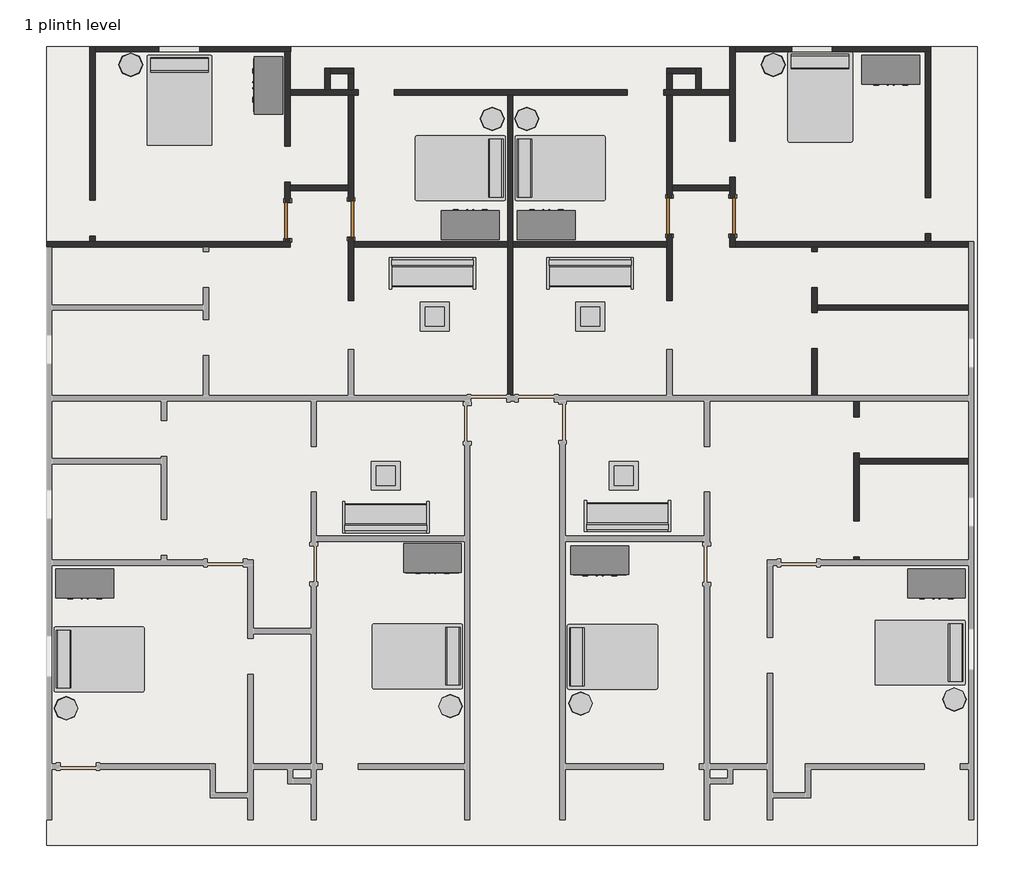
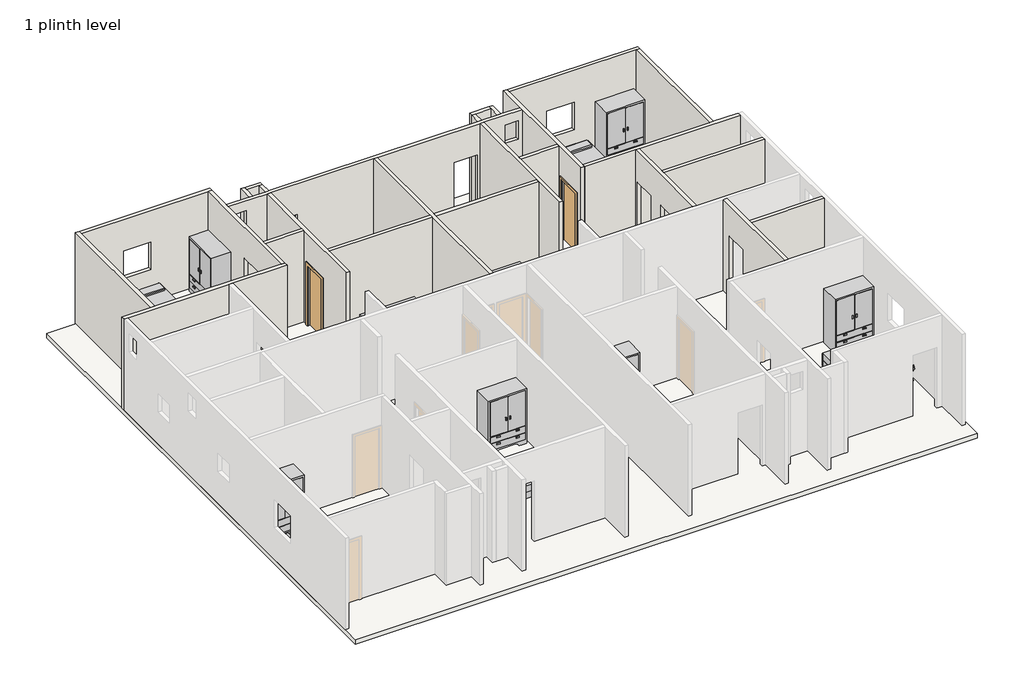
# One storey, part 2 of 2: 32 furniture elements, 26 walls, 4 doors, 1 slab.
"""IFC4 building model written with IfcOpenShell, lengths in millimetres."""

from ifc_helpers import new_model, si_unit, frame, origin, place, context, project, spatial, polyline, outline, extrude, faceted_brep, transform, mapped, element, save
from components import door_f2b275c1, door_d8f5dbb5, furniture_52ef1662, furniture_57f9710a, furniture_d3665cec, furniture_9d41381f, furniture_82e269c4

model = new_model("IFC4")

# Units and contexts
model_context = context("Model", 3, world=origin())
ifc_project = project(units=[si_unit("LENGTHUNIT", "METRE", prefix="MILLI")], contexts=[model_context])

# Site, building, storey
site = spatial("IfcSite", under=ifc_project)
building = spatial("IfcBuilding", under=site)
storey = spatial("IfcBuildingStorey", under=building, Name="1 plinth level", Elevation=457.2)

# Doors
placement = place(None, origin())
door_shape = door_f2b275c1(model_context)
element("IfcDoor", 1, ObjectType="Single-Flush : 30\" x 80\"", at=placement, inside=storey, context=model_context, shape_type="MappedRepresentation", body=[
    mapped(door_shape, transform((-9758.6269874, 1511.4935601, 457.2), x_axis=(0.0, -1.0, 0.0), y_axis=(1.0, 0.0, 0.0), z_axis=(0.0, 0.0, 1.0))),
])
element("IfcDoor", 2, ObjectType="Single-Flush : 30\" x 80\"", at=placement, inside=storey, context=model_context, shape_type="MappedRepresentation", body=[
    mapped(door_shape, transform((-1689.6343188, 1600.3935601, 457.2), x_axis=(0.0, -1.0, 0.0), y_axis=(1.0, 0.0, 0.0), z_axis=(0.0, 0.0, 1.0))),
])
door_2_shape = door_d8f5dbb5(model_context)
element("IfcDoor", 3, ObjectType="Single-Flush : 30\" x 80\"", at=placement, inside=storey, context=model_context, shape_type="MappedRepresentation", body=[
    mapped(door_2_shape, transform((-8420.6343188, 1536.8935601, 457.2), x_axis=(0.0, -1.0, 0.0), y_axis=(1.0, 0.0, 0.0), z_axis=(0.0, 0.0, 1.0))),
])
element("IfcDoor", 4, ObjectType="Single-Flush : 30\" x 80\"", at=placement, inside=storey, context=model_context, shape_type="MappedRepresentation", body=[
    mapped(door_2_shape, transform((-356.1343188, 1600.3935601, 457.2), x_axis=(0.0, -1.0, 0.0), y_axis=(1.0, 0.0, 0.0), z_axis=(0.0, 0.0, 1.0))),
])

# Furniture
furniture_shape = furniture_52ef1662(model_context)
element("IfcFurniture", 5, ObjectType="Bed-Standard : Double 54\" x 75\"", at=placement, inside=storey, context=model_context, shape_type="MappedRepresentation", body=[
    mapped(furniture_shape, transform((-12316.115512, 4097.0886421, 457.2), x_axis=(1.0, 0.0, 0.0), y_axis=(0.0, 1.0, 0.0), z_axis=(0.0, 0.0, 1.0))),
])
element("IfcFurniture", 6, ObjectType="Bed-Standard : Double 54\" x 75\"", at=placement, inside=storey, context=model_context, shape_type="MappedRepresentation", body=[
    mapped(furniture_shape, transform((-6063.6392368, 2886.3142767, 457.2), x_axis=(0.0, -1.0, 0.0), y_axis=(1.0, 0.0, 0.0), z_axis=(0.0, 0.0, 1.0))),
])
element("IfcFurniture", 7, ObjectType="Bed-Standard : Double 54\" x 75\"", at=placement, inside=storey, context=model_context, shape_type="MappedRepresentation", body=[
    mapped(furniture_shape, transform((-4046.6294008, 2343.3372275, 457.2), x_axis=(0.0, 1.0, 0.0), y_axis=(-1.0, 0.0, 0.0), z_axis=(0.0, 0.0, 1.0))),
])
element("IfcFurniture", 8, ObjectType="Bed-Standard : Double 54\" x 75\"", at=placement, inside=storey, context=model_context, shape_type="MappedRepresentation", body=[
    mapped(furniture_shape, transform((1220.2271566, 4166.9386421, 457.2), x_axis=(1.0, 0.0, 0.0), y_axis=(0.0, 1.0, 0.0), z_axis=(0.0, 0.0, 1.0))),
])
element("IfcFurniture", 9, ObjectType="Bed-Standard : Double 54\" x 75\"", at=placement, inside=storey, context=model_context, shape_type="MappedRepresentation", body=[
    mapped(furniture_shape, transform((-13787.5294008, -8037.3449645, 457.2), x_axis=(0.0, 1.0, 0.0), y_axis=(-1.0, 0.0, 0.0), z_axis=(0.0, 0.0, 1.0))),
])
element("IfcFurniture", 10, ObjectType="Bed-Standard : Double 54\" x 75\"", at=placement, inside=storey, context=model_context, shape_type="MappedRepresentation", body=[
    mapped(furniture_shape, transform((-6972.9182387, -7430.8679153, 457.2), x_axis=(0.0, -1.0, 0.0), y_axis=(1.0, 0.0, 0.0), z_axis=(0.0, 0.0, 1.0))),
])
element("IfcFurniture", 11, ObjectType="Bed-Standard : Double 54\" x 75\"", at=placement, inside=storey, context=model_context, shape_type="MappedRepresentation", body=[
    mapped(furniture_shape, transform((-2941.8986045, -7986.5449645, 457.2), x_axis=(0.0, 1.0, 0.0), y_axis=(-1.0, 0.0, 0.0), z_axis=(0.0, 0.0, 1.0))),
])
element("IfcFurniture", 12, ObjectType="Bed-Standard : Double 54\" x 75\"", at=placement, inside=storey, context=model_context, shape_type="MappedRepresentation", body=[
    mapped(furniture_shape, transform((3651.8607632, -7354.6679153, 457.2), x_axis=(0.0, -1.0, 0.0), y_axis=(1.0, 0.0, 0.0), z_axis=(0.0, 0.0, 1.0))),
])
furniture_2_shape = furniture_57f9710a(model_context)
element("IfcFurniture", 13, ObjectType="Sofa : 72\"", at=placement, inside=storey, context=model_context, shape_type="MappedRepresentation", body=[
    mapped(furniture_2_shape, transform((-6771.3838124, 247.7394618, 457.2), x_axis=(1.0, 0.0, 0.0), y_axis=(0.0, 1.0, 0.0), z_axis=(0.0, 0.0, 1.0))),
])
element("IfcFurniture", 14, ObjectType="Sofa : 72\"", at=placement, inside=storey, context=model_context, shape_type="MappedRepresentation", body=[
    mapped(furniture_2_shape, transform((-3436.4048106, 247.7394618, 457.2), x_axis=(1.0, 0.0, 0.0), y_axis=(0.0, 1.0, 0.0), z_axis=(0.0, 0.0, 1.0))),
])
element("IfcFurniture", 15, ObjectType="Sofa : 72\"", at=placement, inside=storey, context=model_context, shape_type="MappedRepresentation", body=[
    mapped(furniture_2_shape, transform((-7613.663827, -4616.1523415, 457.2), x_axis=(-1.0, 0.0, 0.0), y_axis=(0.0, -1.0, 0.0), z_axis=(0.0, 0.0, 1.0))),
])
element("IfcFurniture", 16, ObjectType="Sofa : 72\"", at=placement, inside=storey, context=model_context, shape_type="MappedRepresentation", body=[
    mapped(furniture_2_shape, transform((-2508.4330307, -4590.7523415, 457.2), x_axis=(-1.0, 0.0, 0.0), y_axis=(0.0, -1.0, 0.0), z_axis=(0.0, 0.0, 1.0))),
])
furniture_3_shape = furniture_d3665cec(model_context)
element("IfcFurniture", 17, ObjectType="Table-Coffee : 24\" x 24\" x 24\"", at=placement, inside=storey, context=model_context, shape_type="MappedRepresentation", body=[
    mapped(furniture_3_shape, transform((-6668.4790873, -615.7175177, 457.2), x_axis=(1.0, 0.0, 0.0), y_axis=(0.0, 1.0, 0.0), z_axis=(0.0, 0.0, 1.0))),
])
element("IfcFurniture", 18, ObjectType="Table-Coffee : 24\" x 24\" x 24\"", at=placement, inside=storey, context=model_context, shape_type="MappedRepresentation", body=[
    mapped(furniture_3_shape, transform((-3384.3000855, -615.7175177, 457.2), x_axis=(1.0, 0.0, 0.0), y_axis=(0.0, 1.0, 0.0), z_axis=(0.0, 0.0, 1.0))),
])
element("IfcFurniture", 19, ObjectType="Table-Coffee : 24\" x 24\" x 24\"", at=placement, inside=storey, context=model_context, shape_type="MappedRepresentation", body=[
    mapped(furniture_3_shape, transform((-7702.3000855, -3981.2175177, 457.2), x_axis=(1.0, 0.0, 0.0), y_axis=(0.0, 1.0, 0.0), z_axis=(0.0, 0.0, 1.0))),
])
element("IfcFurniture", 20, ObjectType="Table-Coffee : 24\" x 24\" x 24\"", at=placement, inside=storey, context=model_context, shape_type="MappedRepresentation", body=[
    mapped(furniture_3_shape, transform((-2673.1000855, -3981.2175177, 457.2), x_axis=(1.0, 0.0, 0.0), y_axis=(0.0, 1.0, 0.0), z_axis=(0.0, 0.0, 1.0))),
])
furniture_4_shape = furniture_9d41381f(model_context)
element("IfcFurniture", 21, ObjectType="Table-Trio End : 20\" Diameter", at=placement, inside=storey, context=model_context, shape_type="MappedRepresentation", body=[
    mapped(furniture_4_shape, transform((-13075.1843188, 4800.7935601, 457.2), x_axis=(1.0, 0.0, 0.0), y_axis=(0.0, 1.0, 0.0), z_axis=(0.0, 0.0, 1.0))),
])
element("IfcFurniture", 22, ObjectType="Table-Trio End : 20\" Diameter", at=placement, inside=storey, context=model_context, shape_type="MappedRepresentation", body=[
    mapped(furniture_4_shape, transform((-5436.1343188, 3657.7935601, 457.2), x_axis=(1.0, 0.0, 0.0), y_axis=(0.0, 1.0, 0.0), z_axis=(0.0, 0.0, 1.0))),
])
element("IfcFurniture", 23, ObjectType="Table-Trio End : 20\" Diameter", at=placement, inside=storey, context=model_context, shape_type="MappedRepresentation", body=[
    mapped(furniture_4_shape, transform((-4706.6059618, 3657.7935601, 457.2), x_axis=(1.0, 0.0, 0.0), y_axis=(0.0, 1.0, 0.0), z_axis=(0.0, 0.0, 1.0))),
])
element("IfcFurniture", 24, ObjectType="Table-Trio End : 20\" Diameter", at=placement, inside=storey, context=model_context, shape_type="MappedRepresentation", body=[
    mapped(furniture_4_shape, transform((501.1156812, 4800.7935601, 457.2), x_axis=(1.0, 0.0, 0.0), y_axis=(0.0, 1.0, 0.0), z_axis=(0.0, 0.0, 1.0))),
])
element("IfcFurniture", 25, ObjectType="Table-Trio End : 20\" Diameter", at=placement, inside=storey, context=model_context, shape_type="MappedRepresentation", body=[
    mapped(furniture_4_shape, transform((4330.1656812, -8616.7564399, 457.2), x_axis=(1.0, 0.0, 0.0), y_axis=(0.0, 1.0, 0.0), z_axis=(0.0, 0.0, 1.0))),
])
element("IfcFurniture", 26, ObjectType="Table-Trio End : 20\" Diameter", at=placement, inside=storey, context=model_context, shape_type="MappedRepresentation", body=[
    mapped(furniture_4_shape, transform((-3569.2343188, -8702.0106007, 457.2), x_axis=(1.0, 0.0, 0.0), y_axis=(0.0, 1.0, 0.0), z_axis=(0.0, 0.0, 1.0))),
])
element("IfcFurniture", 27, ObjectType="Table-Trio End : 20\" Diameter", at=placement, inside=storey, context=model_context, shape_type="MappedRepresentation", body=[
    mapped(furniture_4_shape, transform((-6320.0133206, -8756.4564399, 457.2), x_axis=(1.0, 0.0, 0.0), y_axis=(0.0, 1.0, 0.0), z_axis=(0.0, 0.0, 1.0))),
])
element("IfcFurniture", 28, ObjectType="Table-Trio End : 20\" Diameter", at=placement, inside=storey, context=model_context, shape_type="MappedRepresentation", body=[
    mapped(furniture_4_shape, transform((-14440.4343188, -8800.9064399, 457.2), x_axis=(1.0, 0.0, 0.0), y_axis=(0.0, 1.0, 0.0), z_axis=(0.0, 0.0, 1.0))),
])
furniture_5_shape = furniture_82e269c4(model_context)
element("IfcFurniture", 29, ObjectType="Wardrobe : 48\" x 72\" x 24\"", at=placement, inside=storey, context=model_context, shape_type="MappedRepresentation", body=[
    mapped(furniture_5_shape, transform((-9581.2881778, 4098.2324922, 457.2), x_axis=(0.0, -1.0, 0.0), y_axis=(1.0, 0.0, 0.0), z_axis=(0.0, 0.0, 1.0))),
])
element("IfcFurniture", 30, ObjectType="Wardrobe : 48\" x 72\" x 24\"", at=placement, inside=storey, context=model_context, shape_type="MappedRepresentation", body=[
    mapped(furniture_5_shape, transform((-6168.8775786, 826.1547505, 457.2), x_axis=(-1.0, 0.0, 0.0), y_axis=(0.0, -1.0, 0.0), z_axis=(0.0, 0.0, 1.0))),
])
element("IfcFurniture", 31, ObjectType="Wardrobe : 48\" x 72\" x 24\"", at=placement, inside=storey, context=model_context, shape_type="MappedRepresentation", body=[
    mapped(furniture_5_shape, transform((-4562.3275786, 826.1547505, 457.2), x_axis=(-1.0, 0.0, 0.0), y_axis=(0.0, -1.0, 0.0), z_axis=(0.0, 0.0, 1.0))),
])
element("IfcFurniture", 32, ObjectType="Wardrobe : 48\" x 72\" x 24\"", at=placement, inside=storey, context=model_context, shape_type="MappedRepresentation", body=[
    mapped(furniture_5_shape, transform((3253.158941, 5282.9323697, 457.2), x_axis=(1.0, 0.0, 0.0), y_axis=(0.0, 1.0, 0.0), z_axis=(0.0, 0.0, 1.0))),
])
element("IfcFurniture", 33, ObjectType="Wardrobe : 48\" x 72\" x 24\"", at=placement, inside=storey, context=model_context, shape_type="MappedRepresentation", body=[
    mapped(furniture_5_shape, transform((4218.358941, -5575.5676303, 457.2), x_axis=(1.0, 0.0, 0.0), y_axis=(0.0, 1.0, 0.0), z_axis=(0.0, 0.0, 1.0))),
])
element("IfcFurniture", 34, ObjectType="Wardrobe : 48\" x 72\" x 24\"", at=placement, inside=storey, context=model_context, shape_type="MappedRepresentation", body=[
    mapped(furniture_5_shape, transform((-2893.641059, -5086.6176303, 457.2), x_axis=(1.0, 0.0, 0.0), y_axis=(0.0, 1.0, 0.0), z_axis=(0.0, 0.0, 1.0))),
])
element("IfcFurniture", 35, ObjectType="Wardrobe : 48\" x 72\" x 24\"", at=placement, inside=storey, context=model_context, shape_type="MappedRepresentation", body=[
    mapped(furniture_5_shape, transform((-6431.8200608, -5042.1676303, 457.2), x_axis=(1.0, 0.0, 0.0), y_axis=(0.0, 1.0, 0.0), z_axis=(0.0, 0.0, 1.0))),
])
element("IfcFurniture", 36, ObjectType="Wardrobe : 48\" x 72\" x 24\"", at=placement, inside=storey, context=model_context, shape_type="MappedRepresentation", body=[
    mapped(furniture_5_shape, transform((-13777.541059, -5575.5676303, 457.2), x_axis=(1.0, 0.0, 0.0), y_axis=(0.0, 1.0, 0.0), z_axis=(0.0, 0.0, 1.0))),
])

# Slab
element("IfcSlab", 37, ObjectType="6\"", at=placement, inside=storey, context=model_context, shape_type="SweptSolid", body=[
    extrude(outline(polyline([(-14853.1843188, -11697.2008638), (-14853.1843188, 5188.1435601), (4816.0294854, 5188.1435601), (4816.0294854, -11697.2008638), (-14853.1843188, -11697.2008638)])), frame((0.0, 0.0, 304.8), z_axis=(0.0, 0.0, 1.0), x_axis=(1.0, 0.0, 0.0)), (0.0, 0.0, 1.0), 152.4),
])

# Walls
element("IfcWall", 38, ObjectType="wall-4.5\"", at=placement, inside=storey, context=model_context, shape_type="Brep", body=[
    faceted_brep([(-13824.4843188, 5073.8435601, 457.2), (-9815.7769874, 5073.8435601, 457.2), (-9701.4769874, 5073.8435601, 457.2), (-9696.9843188, 5073.8435601, 457.2), (-9696.9843188, 5073.8435601, 3505.2), (-9701.4769874, 5073.8435601, 3505.2), (-9815.7769874, 5073.8435601, 3505.2), (-13824.4843188, 5073.8435601, 3505.2), (-11621.0343188, 5073.8435601, 2438.4), (-11621.0343188, 5073.8435601, 1524.0), (-12484.6343188, 5073.8435601, 1524.0), (-12484.6343188, 5073.8435601, 2438.4), (-13824.4843188, 5188.1435601, 457.2), (-13824.4843188, 5188.1435601, 3505.2), (-9696.9843188, 5188.1435601, 3505.2), (-9696.9843188, 5188.1435601, 457.2), (-11621.0343188, 5188.1435601, 2438.4), (-12484.6343188, 5188.1435601, 2438.4), (-12484.6343188, 5188.1435601, 1524.0), (-11621.0343188, 5188.1435601, 1524.0)], [[[0, 1, 2, 3, 4, 5, 6, 7], [8, 9, 10, 11]], [[12, 13, 14, 15], [16, 17, 18, 19]], [[3, 2, 1, 0, 12, 15]], [[4, 3, 15, 14]], [[7, 6, 5, 4, 14, 13]], [[0, 7, 13, 12]], [[9, 8, 16, 19]], [[10, 9, 19, 18]], [[11, 10, 18, 17]], [[8, 11, 17, 16]]]),
])
element("IfcWall", 39, ObjectType="wall-4.5\"", at=placement, inside=storey, context=model_context, shape_type="Brep", body=[
    faceted_brep([(-9815.7769874, 2324.2935601, 2489.2), (-9815.7769874, 2324.2935601, 457.2), (-9815.7769874, 1892.4935601, 457.2), (-9815.7769874, 1892.4935601, 2489.2), (-9815.7769874, 1130.4935601, 2489.2), (-9815.7769874, 1130.4935601, 457.2), (-9815.7769874, 1060.6435601, 457.2), (-9815.7769874, 1060.6435601, 3505.2), (-9815.7769874, 5073.8435601, 3505.2), (-9815.7769874, 5073.8435601, 457.2), (-9815.7769874, 3086.2935601, 457.2), (-9815.7769874, 3086.2935601, 2489.2), (-9701.4769874, 1892.4935601, 457.2), (-9701.4769874, 2140.1435601, 457.2), (-9701.4769874, 2254.4435601, 457.2), (-9701.4769874, 2324.2935601, 457.2), (-9701.4769874, 2324.2935601, 2489.2), (-9701.4769874, 3086.2935601, 2489.2), (-9701.4769874, 3086.2935601, 457.2), (-9701.4769874, 4159.4435601, 457.2), (-9701.4769874, 4273.7435601, 457.2), (-9701.4769874, 5073.8435601, 457.2), (-9701.4769874, 5073.8435601, 3505.2), (-9701.4769874, 4273.7435601, 3505.2), (-9701.4769874, 4159.4435601, 3505.2), (-9701.4769874, 2254.4435601, 3505.2), (-9701.4769874, 2140.1435601, 3505.2), (-9701.4769874, 1060.6435601, 3505.2), (-9701.4769874, 1060.6435601, 457.2), (-9701.4769874, 1130.4935601, 457.2), (-9701.4769874, 1130.4935601, 2489.2), (-9701.4769874, 1892.4935601, 2489.2)], [[[0, 1, 2, 3, 4, 5, 6, 7, 8, 9, 10, 11]], [[12, 13, 14, 15, 16, 17, 18, 19, 20, 21, 22, 23, 24, 25, 26, 27, 28, 29, 30, 31]], [[28, 6, 5, 29]], [[10, 9, 21, 20, 19, 18]], [[2, 1, 15, 14, 13, 12]], [[8, 7, 27, 26, 25, 24, 23, 22]], [[7, 6, 28, 27]], [[9, 8, 22, 21]], [[4, 30, 29, 5]], [[30, 4, 3, 31]], [[31, 3, 2, 12]], [[16, 15, 1, 0]], [[17, 16, 0, 11]], [[18, 17, 11, 10]]]),
])
element("IfcWall", 40, ObjectType="wall-4.5\"", at=placement, inside=storey, context=model_context, shape_type="Brep", body=[
    faceted_brep([(-9701.4769874, 1060.6435601, 457.2), (-9815.7769874, 1060.6435601, 457.2), (-13824.4843188, 1060.6435601, 457.2), (-13938.7843188, 1060.6435601, 457.2), (-14853.1843188, 1060.6435601, 457.2), (-14853.1843188, 1060.6435601, 3505.2), (-13938.7843188, 1060.6435601, 3505.2), (-13824.4843188, 1060.6435601, 3505.2), (-9815.7769874, 1060.6435601, 3505.2), (-9701.4769874, 1060.6435601, 3505.2), (-9701.4769874, 946.3435601, 457.2), (-9701.4769874, 946.3435601, 3505.2), (-11424.1843188, 946.3435601, 3505.2), (-11538.4843188, 946.3435601, 3505.2), (-14738.8843188, 946.3435601, 3505.2), (-14853.1843188, 946.3435601, 3505.2), (-14853.1843188, 946.3435601, 457.2), (-14738.8843188, 946.3435601, 457.2), (-11538.4843188, 946.3435601, 457.2), (-11424.1843188, 946.3435601, 457.2)], [[[0, 1, 2, 3, 4, 5, 6, 7, 8, 9]], [[10, 11, 12, 13, 14, 15, 16, 17, 18, 19]], [[4, 3, 2, 1, 0, 10, 19, 18, 17, 16]], [[9, 8, 7, 6, 5, 15, 14, 13, 12, 11]], [[0, 9, 11, 10]], [[5, 4, 16, 15]]]),
])
element("IfcWall", 41, ObjectType="wall-4.5\"", at=placement, inside=storey, context=model_context, shape_type="Brep", body=[
    faceted_brep([(-13938.7843188, 1181.2935601, 2489.2), (-13938.7843188, 1181.2935601, 457.2), (-13938.7843188, 1060.6435601, 457.2), (-13938.7843188, 1060.6435601, 3505.2), (-13938.7843188, 5188.1435601, 3505.2), (-13938.7843188, 5188.1435601, 457.2), (-13938.7843188, 1943.2935601, 457.2), (-13938.7843188, 1943.2935601, 2489.2), (-13824.4843188, 1060.6435601, 457.2), (-13824.4843188, 1181.2935601, 457.2), (-13824.4843188, 1181.2935601, 2489.2), (-13824.4843188, 1943.2935601, 2489.2), (-13824.4843188, 1943.2935601, 457.2), (-13824.4843188, 5073.8435601, 457.2), (-13824.4843188, 5188.1435601, 457.2), (-13824.4843188, 5188.1435601, 3505.2), (-13824.4843188, 5073.8435601, 3505.2), (-13824.4843188, 1060.6435601, 3505.2)], [[[0, 1, 2, 3, 4, 5, 6, 7]], [[8, 9, 10, 11, 12, 13, 14, 15, 16, 17]], [[6, 5, 14, 13, 12]], [[2, 1, 9, 8]], [[4, 3, 17, 16, 15]], [[3, 2, 8, 17]], [[5, 4, 15, 14]], [[10, 9, 1, 0]], [[11, 10, 0, 7]], [[12, 11, 7, 6]]]),
])
element("IfcWall", 42, ObjectType="wall-4.5\"", at=placement, inside=storey, context=model_context, shape_type="Brep", body=[
    faceted_brep([(-9701.4769874, 4159.4435601, 457.2), (-8477.7843188, 4159.4435601, 457.2), (-8363.4843188, 4159.4435601, 457.2), (-8266.3769874, 4159.4435601, 457.2), (-8266.3769874, 4159.4435601, 2489.2), (-7504.3769874, 4159.4435601, 2489.2), (-7504.3769874, 4159.4435601, 457.2), (-5112.2843188, 4159.4435601, 457.2), (-4997.9843188, 4159.4435601, 457.2), (-2578.6343188, 4159.4435601, 457.2), (-2578.6343188, 4159.4435601, 2489.2), (-1816.6343188, 4159.4435601, 2489.2), (-1816.6343188, 4159.4435601, 457.2), (-1746.7843188, 4159.4435601, 457.2), (-1632.4843188, 4159.4435601, 457.2), (-414.0059618, 4159.4435601, 457.2), (-414.0059618, 4159.4435601, 3505.2), (-1632.4843188, 4159.4435601, 3505.2), (-1746.7843188, 4159.4435601, 3505.2), (-4997.9843188, 4159.4435601, 3505.2), (-5112.2843188, 4159.4435601, 3505.2), (-8363.4843188, 4159.4435601, 3505.2), (-8477.7843188, 4159.4435601, 3505.2), (-9701.4769874, 4159.4435601, 3505.2), (-9134.0806531, 4159.4435601, 3175.0), (-9134.0806531, 4159.4435601, 2565.4), (-9540.4806531, 4159.4435601, 2565.4), (-9540.4806531, 4159.4435601, 3175.0), (-543.8201403, 4159.4435601, 3175.0), (-543.8201403, 4159.4435601, 2565.4), (-950.2201403, 4159.4435601, 2565.4), (-950.2201403, 4159.4435601, 3175.0), (-8266.3769874, 4273.7435601, 2489.2), (-8266.3769874, 4273.7435601, 457.2), (-8361.6269874, 4273.7435601, 457.2), (-8475.9269874, 4273.7435601, 457.2), (-8858.7843188, 4273.7435601, 457.2), (-8973.0843188, 4273.7435601, 457.2), (-9701.4769874, 4273.7435601, 457.2), (-9701.4769874, 4273.7435601, 3505.2), (-8973.0843188, 4273.7435601, 3505.2), (-8858.7843188, 4273.7435601, 3505.2), (-8475.9269874, 4273.7435601, 3505.2), (-8361.6269874, 4273.7435601, 3505.2), (-1746.7843188, 4273.7435601, 3505.2), (-1632.4843188, 4273.7435601, 3505.2), (-1137.1843188, 4273.7435601, 3505.2), (-1022.8843188, 4273.7435601, 3505.2), (-414.0059618, 4273.7435601, 3505.2), (-414.0059618, 4273.7435601, 457.2), (-1022.8843188, 4273.7435601, 457.2), (-1137.1843188, 4273.7435601, 457.2), (-1632.4843188, 4273.7435601, 457.2), (-1746.7843188, 4273.7435601, 457.2), (-1816.6343188, 4273.7435601, 457.2), (-1816.6343188, 4273.7435601, 2489.2), (-2578.6343188, 4273.7435601, 2489.2), (-2578.6343188, 4273.7435601, 457.2), (-7504.3769874, 4273.7435601, 457.2), (-7504.3769874, 4273.7435601, 2489.2), (-9134.0806531, 4273.7435601, 3175.0), (-9540.4806531, 4273.7435601, 3175.0), (-9540.4806531, 4273.7435601, 2565.4), (-9134.0806531, 4273.7435601, 2565.4), (-543.8201403, 4273.7435601, 3175.0), (-950.2201403, 4273.7435601, 3175.0), (-950.2201403, 4273.7435601, 2565.4), (-543.8201403, 4273.7435601, 2565.4)], [[[0, 1, 2, 3, 4, 5, 6, 7, 8, 9, 10, 11, 12, 13, 14, 15, 16, 17, 18, 19, 20, 21, 22, 23], [24, 25, 26, 27], [28, 29, 30, 31]], [[32, 33, 34, 35, 36, 37, 38, 39, 40, 41, 42, 43, 44, 45, 46, 47, 48, 49, 50, 51, 52, 53, 54, 55, 56, 57, 58, 59], [60, 61, 62, 63], [64, 65, 66, 67]], [[15, 14, 13, 12, 54, 53, 52, 51, 50, 49]], [[58, 57, 9, 8, 7, 6]], [[38, 37, 36, 35, 34, 33, 3, 2, 1, 0]], [[16, 15, 49, 48]], [[23, 22, 21, 20, 19, 18, 17, 16, 48, 47, 46, 45, 44, 43, 42, 41, 40, 39]], [[0, 23, 39, 38]], [[55, 54, 12, 11]], [[56, 55, 11, 10]], [[57, 56, 10, 9]], [[4, 3, 33, 32]], [[5, 4, 32, 59]], [[6, 5, 59, 58]], [[25, 24, 60, 63]], [[26, 25, 63, 62]], [[27, 26, 62, 61]], [[24, 27, 61, 60]], [[29, 28, 64, 67]], [[30, 29, 67, 66]], [[31, 30, 66, 65]], [[28, 31, 65, 64]]]),
])
element("IfcWall", 43, ObjectType="wall-4.5\"", at=placement, inside=storey, context=model_context, shape_type="Brep", body=[
    faceted_brep([(-8858.7843188, 4273.7435601, 457.2), (-8858.7843188, 4616.6435601, 457.2), (-8858.7843188, 4730.9435601, 457.2), (-8858.7843188, 4730.9435601, 3505.2), (-8858.7843188, 4616.6435601, 3505.2), (-8858.7843188, 4273.7435601, 3505.2), (-8973.0843188, 4273.7435601, 457.2), (-8973.0843188, 4273.7435601, 3505.2), (-8973.0843188, 4730.9435601, 3505.2), (-8973.0843188, 4730.9435601, 457.2)], [[[0, 1, 2, 3, 4, 5]], [[6, 7, 8, 9]], [[2, 1, 0, 6, 9]], [[5, 4, 3, 8, 7]], [[0, 5, 7, 6]], [[3, 2, 9, 8]]]),
])
element("IfcWall", 44, ObjectType="wall-4.5\"", at=placement, inside=storey, context=model_context, shape_type="SweptSolid", body=[
    extrude(outline(polyline([(-8361.6269874, 4616.6435601), (-8361.6269874, 4273.7435601), (-8475.9269874, 4273.7435601), (-8475.9269874, 4616.6435601), (-8361.6269874, 4616.6435601)])), frame((0.0, 0.0, 457.2), z_axis=(0.0, 0.0, 1.0), x_axis=(1.0, 0.0, 0.0)), (0.0, 0.0, 1.0), 3048.0),
])
element("IfcWall", 45, ObjectType="wall-4.5\"", at=placement, inside=storey, context=model_context, shape_type="Brep", body=[
    faceted_brep([(-8361.6269874, 4730.9435601, 457.2), (-8858.7843188, 4730.9435601, 457.2), (-8858.7843188, 4730.9435601, 3505.2), (-8361.6269874, 4730.9435601, 3505.2), (-8361.6269874, 4616.6435601, 457.2), (-8361.6269874, 4616.6435601, 3505.2), (-8475.9269874, 4616.6435601, 3505.2), (-8858.7843188, 4616.6435601, 3505.2), (-8858.7843188, 4616.6435601, 457.2), (-8475.9269874, 4616.6435601, 457.2)], [[[0, 1, 2, 3]], [[4, 5, 6, 7, 8, 9]], [[1, 0, 4, 9, 8]], [[3, 2, 7, 6, 5]], [[2, 1, 8, 7]], [[0, 3, 5, 4]]]),
])
element("IfcWall", 46, ObjectType="wall-4.5\"", at=placement, inside=storey, context=model_context, shape_type="Brep", body=[
    faceted_brep([(-8477.7843188, -179.1742479, 457.2), (-8477.7843188, -179.1742479, 3505.2), (-8477.7843188, 2140.1435601, 3505.2), (-8477.7843188, 2254.4435601, 3505.2), (-8477.7843188, 4159.4435601, 3505.2), (-8477.7843188, 4159.4435601, 457.2), (-8477.7843188, 2254.4435601, 457.2), (-8477.7843188, 2140.1435601, 457.2), (-8477.7843188, 1917.8935601, 457.2), (-8477.7843188, 1917.8935601, 2489.2), (-8477.7843188, 1155.8935601, 2489.2), (-8477.7843188, 1155.8935601, 457.2), (-8363.4843188, -179.1742479, 3505.2), (-8363.4843188, -179.1742479, 457.2), (-8363.4843188, 946.3435601, 457.2), (-8363.4843188, 1060.6435601, 457.2), (-8363.4843188, 1155.8935601, 457.2), (-8363.4843188, 1155.8935601, 2489.2), (-8363.4843188, 1917.8935601, 2489.2), (-8363.4843188, 1917.8935601, 457.2), (-8363.4843188, 4159.4435601, 457.2), (-8363.4843188, 4159.4435601, 3505.2), (-8363.4843188, 1060.6435601, 3505.2), (-8363.4843188, 946.3435601, 3505.2)], [[[0, 1, 2, 3, 4, 5, 6, 7, 8, 9, 10, 11]], [[12, 13, 14, 15, 16, 17, 18, 19, 20, 21, 22, 23]], [[13, 0, 11, 16, 15, 14]], [[5, 20, 19, 8, 7, 6]], [[1, 0, 13, 12]], [[4, 3, 2, 1, 12, 23, 22, 21]], [[5, 4, 21, 20]], [[10, 17, 16, 11]], [[17, 10, 9, 18]], [[18, 9, 8, 19]]]),
])
element("IfcWall", 47, ObjectType="wall-4.5\"", at=placement, inside=storey, context=model_context, shape_type="Brep", body=[
    faceted_brep([(-413.2843188, 5188.1435601, 457.2), (-413.2843188, 3187.8935601, 457.2), (-413.2843188, 3187.8935601, 2489.2), (-413.2843188, 2425.8935601, 2489.2), (-413.2843188, 2425.8935601, 457.2), (-413.2843188, 2254.4435601, 457.2), (-413.2843188, 2140.1435601, 457.2), (-413.2843188, 1981.3935601, 457.2), (-413.2843188, 1981.3935601, 2489.2), (-413.2843188, 1219.3935601, 2489.2), (-413.2843188, 1219.3935601, 457.2), (-413.2843188, 946.3435601, 457.2), (-413.2843188, 946.3435601, 3505.2), (-413.2843188, 2140.1435601, 3505.2), (-413.2843188, 2254.4435601, 3505.2), (-413.2843188, 5188.1435601, 3505.2), (-298.9843188, 3187.8935601, 2489.2), (-298.9843188, 3187.8935601, 457.2), (-298.9843188, 5073.8435601, 457.2), (-298.9843188, 5188.1435601, 457.2), (-298.9843188, 5188.1435601, 3505.2), (-298.9843188, 5073.8435601, 3505.2), (-298.9843188, 1060.6435601, 3505.2), (-298.9843188, 946.3435601, 3505.2), (-298.9843188, 946.3435601, 457.2), (-298.9843188, 1060.6435601, 457.2), (-298.9843188, 1219.3935601, 457.2), (-298.9843188, 1219.3935601, 2489.2), (-298.9843188, 1981.3935601, 2489.2), (-298.9843188, 1981.3935601, 457.2), (-298.9843188, 2425.8935601, 457.2), (-298.9843188, 2425.8935601, 2489.2)], [[[0, 1, 2, 3, 4, 5, 6, 7, 8, 9, 10, 11, 12, 13, 14, 15]], [[16, 17, 18, 19, 20, 21, 22, 23, 24, 25, 26, 27, 28, 29, 30, 31]], [[24, 11, 10, 26, 25]], [[30, 29, 7, 6, 5, 4]], [[19, 18, 17, 1, 0]], [[15, 14, 13, 12, 23, 22, 21, 20]], [[12, 11, 24, 23]], [[0, 15, 20, 19]], [[9, 27, 26, 10]], [[27, 9, 8, 28]], [[28, 8, 7, 29]], [[2, 1, 17, 16]], [[3, 2, 16, 31]], [[4, 3, 31, 30]]]),
])
element("IfcWall", 48, ObjectType="wall-4.5\"", at=placement, inside=storey, context=model_context, shape_type="Brep", body=[
    faceted_brep([(-298.9843188, 946.3435601, 457.2), (1313.9156812, 946.3435601, 457.2), (1428.2156812, 946.3435601, 457.2), (4628.6156812, 946.3435601, 457.2), (4628.6156812, 946.3435601, 3505.2), (1428.2156812, 946.3435601, 3505.2), (1313.9156812, 946.3435601, 3505.2), (-298.9843188, 946.3435601, 3505.2), (-298.9843188, 1060.6435601, 457.2), (-298.9843188, 1060.6435601, 3505.2), (3714.2156812, 1060.6435601, 3505.2), (3828.5156812, 1060.6435601, 3505.2), (4628.6156812, 1060.6435601, 3505.2), (4628.6156812, 1060.6435601, 457.2), (3828.5156812, 1060.6435601, 457.2), (3714.2156812, 1060.6435601, 457.2)], [[[0, 1, 2, 3, 4, 5, 6, 7]], [[8, 9, 10, 11, 12, 13, 14, 15]], [[3, 2, 1, 0, 8, 15, 14, 13]], [[7, 6, 5, 4, 12, 11, 10, 9]], [[0, 7, 9, 8]], [[4, 3, 13, 12]]]),
])
element("IfcWall", 49, ObjectType="wall-4.5\"", at=placement, inside=storey, context=model_context, shape_type="Brep", body=[
    faceted_brep([(-298.9843188, 5073.8435601, 457.2), (3714.2156812, 5073.8435601, 457.2), (3828.5156812, 5073.8435601, 457.2), (3828.5156812, 5073.8435601, 3505.2), (3714.2156812, 5073.8435601, 3505.2), (-298.9843188, 5073.8435601, 3505.2), (1752.0656812, 5073.8435601, 2438.4), (1752.0656812, 5073.8435601, 1524.0), (888.4656812, 5073.8435601, 1524.0), (888.4656812, 5073.8435601, 2438.4), (-298.9843188, 5188.1435601, 457.2), (-298.9843188, 5188.1435601, 3505.2), (3828.5156812, 5188.1435601, 3505.2), (3828.5156812, 5188.1435601, 457.2), (1752.0656812, 5188.1435601, 2438.4), (888.4656812, 5188.1435601, 2438.4), (888.4656812, 5188.1435601, 1524.0), (1752.0656812, 5188.1435601, 1524.0)], [[[0, 1, 2, 3, 4, 5], [6, 7, 8, 9]], [[10, 11, 12, 13], [14, 15, 16, 17]], [[2, 1, 0, 10, 13]], [[5, 4, 3, 12, 11]], [[0, 5, 11, 10]], [[3, 2, 13, 12]], [[7, 6, 14, 17]], [[8, 7, 17, 16]], [[9, 8, 16, 15]], [[6, 9, 15, 14]]]),
])
element("IfcWall", 50, ObjectType="wall-4.5\"", at=placement, inside=storey, context=model_context, shape_type="SweptSolid", body=[
    extrude(outline(polyline([(1232.0935601, 2489.2), (1232.0935601, 457.2), (1060.6435601, 457.2), (1060.6435601, 3505.2), (5073.8435601, 3505.2), (5073.8435601, 457.2), (1994.0935601, 457.2), (1994.0935601, 2489.2), (1232.0935601, 2489.2)])), frame((3714.2156812, 0.0, 0.0), z_axis=(1.0, 0.0, 0.0), x_axis=(0.0, 1.0, 0.0)), (0.0, 0.0, 1.0), 114.3),
])
element("IfcWall", 51, ObjectType="wall-4.5\"", at=placement, inside=storey, context=model_context, shape_type="SweptSolid", body=[
    extrude(outline(polyline([(-8477.7843188, 2140.1435601), (-9701.4769874, 2140.1435601), (-9701.4769874, 2254.4435601), (-8477.7843188, 2254.4435601), (-8477.7843188, 2140.1435601)])), frame((0.0, 0.0, 457.2), z_axis=(0.0, 0.0, 1.0), x_axis=(1.0, 0.0, 0.0)), (0.0, 0.0, 1.0), 3048.0),
])
element("IfcWall", 52, ObjectType="wall-4.5\"", at=placement, inside=storey, context=model_context, shape_type="SweptSolid", body=[
    extrude(outline(polyline([(-1632.4843188, 4616.6435601), (-1632.4843188, 4273.7435601), (-1746.7843188, 4273.7435601), (-1746.7843188, 4616.6435601), (-1632.4843188, 4616.6435601)])), frame((0.0, 0.0, 457.2), z_axis=(0.0, 0.0, 1.0), x_axis=(1.0, 0.0, 0.0)), (0.0, 0.0, 1.0), 3048.0),
])
element("IfcWall", 53, ObjectType="wall-4.5\"", at=placement, inside=storey, context=model_context, shape_type="Brep", body=[
    faceted_brep([(-1746.7843188, 4616.6435601, 457.2), (-1632.4843188, 4616.6435601, 457.2), (-1137.1843188, 4616.6435601, 457.2), (-1137.1843188, 4616.6435601, 3505.2), (-1632.4843188, 4616.6435601, 3505.2), (-1746.7843188, 4616.6435601, 3505.2), (-1746.7843188, 4730.9435601, 457.2), (-1746.7843188, 4730.9435601, 3505.2), (-1137.1843188, 4730.9435601, 3505.2), (-1137.1843188, 4730.9435601, 457.2)], [[[0, 1, 2, 3, 4, 5]], [[6, 7, 8, 9]], [[2, 1, 0, 6, 9]], [[5, 4, 3, 8, 7]], [[3, 2, 9, 8]], [[0, 5, 7, 6]]]),
])
element("IfcWall", 54, ObjectType="wall-4.5\"", at=placement, inside=storey, context=model_context, shape_type="Brep", body=[
    faceted_brep([(-1137.1843188, 4730.9435601, 457.2), (-1137.1843188, 4616.6435601, 457.2), (-1137.1843188, 4273.7435601, 457.2), (-1137.1843188, 4273.7435601, 3505.2), (-1137.1843188, 4616.6435601, 3505.2), (-1137.1843188, 4730.9435601, 3505.2), (-1022.8843188, 4730.9435601, 457.2), (-1022.8843188, 4730.9435601, 3505.2), (-1022.8843188, 4273.7435601, 3505.2), (-1022.8843188, 4273.7435601, 457.2)], [[[0, 1, 2, 3, 4, 5]], [[6, 7, 8, 9]], [[2, 1, 0, 6, 9]], [[5, 4, 3, 8, 7]], [[3, 2, 9, 8]], [[0, 5, 7, 6]]]),
])
element("IfcWall", 55, ObjectType="wall-4.5\"", at=placement, inside=storey, context=model_context, shape_type="Brep", body=[
    faceted_brep([(-1746.7843188, -179.1742479, 457.2), (-1746.7843188, -179.1742479, 3505.2), (-1746.7843188, 946.3435601, 3505.2), (-1746.7843188, 1060.6435601, 3505.2), (-1746.7843188, 4159.4435601, 3505.2), (-1746.7843188, 4159.4435601, 457.2), (-1746.7843188, 1981.3935601, 457.2), (-1746.7843188, 1981.3935601, 2489.2), (-1746.7843188, 1219.3935601, 2489.2), (-1746.7843188, 1219.3935601, 457.2), (-1746.7843188, 1060.6435601, 457.2), (-1746.7843188, 946.3435601, 457.2), (-1632.4843188, -179.1742479, 3505.2), (-1632.4843188, -179.1742479, 457.2), (-1632.4843188, 1219.3935601, 457.2), (-1632.4843188, 1219.3935601, 2489.2), (-1632.4843188, 1981.3935601, 2489.2), (-1632.4843188, 1981.3935601, 457.2), (-1632.4843188, 2140.1435601, 457.2), (-1632.4843188, 2254.4435601, 457.2), (-1632.4843188, 4159.4435601, 457.2), (-1632.4843188, 4159.4435601, 3505.2), (-1632.4843188, 2254.4435601, 3505.2), (-1632.4843188, 2140.1435601, 3505.2)], [[[0, 1, 2, 3, 4, 5, 6, 7, 8, 9, 10, 11]], [[12, 13, 14, 15, 16, 17, 18, 19, 20, 21, 22, 23]], [[13, 0, 11, 10, 9, 14]], [[5, 20, 19, 18, 17, 6]], [[1, 0, 13, 12]], [[4, 3, 2, 1, 12, 23, 22, 21]], [[5, 4, 21, 20]], [[8, 15, 14, 9]], [[15, 8, 7, 16]], [[16, 7, 6, 17]]]),
])
element("IfcWall", 56, ObjectType="wall-4.5\"", at=placement, inside=storey, context=model_context, shape_type="SweptSolid", body=[
    extrude(outline(polyline([(-413.2843188, 2140.1435601), (-1632.4843188, 2140.1435601), (-1632.4843188, 2254.4435601), (-413.2843188, 2254.4435601), (-413.2843188, 2140.1435601)])), frame((0.0, 0.0, 457.2), z_axis=(0.0, 0.0, 1.0), x_axis=(1.0, 0.0, 0.0)), (0.0, 0.0, 1.0), 3048.0),
])
element("IfcWall", 57, ObjectType="wall-4.5\"", at=placement, inside=storey, context=model_context, shape_type="Brep", body=[
    faceted_brep([(1313.9156812, 89.0935601, 457.2), (1313.9156812, -431.6064399, 457.2), (1313.9156812, -431.6064399, 2489.2), (1313.9156812, -1193.6064399, 2489.2), (1313.9156812, -1193.6064399, 457.2), (1313.9156812, -2190.5564399, 457.2), (1313.9156812, -2190.5564399, 3505.2), (1313.9156812, 946.3435601, 3505.2), (1313.9156812, 946.3435601, 457.2), (1313.9156812, 851.0935601, 457.2), (1313.9156812, 851.0935601, 2489.2), (1313.9156812, 89.0935601, 2489.2), (1428.2156812, -431.6064399, 2489.2), (1428.2156812, -431.6064399, 457.2), (1428.2156812, -387.1564399, 457.2), (1428.2156812, -272.8564399, 457.2), (1428.2156812, 89.0935601, 457.2), (1428.2156812, 89.0935601, 2489.2), (1428.2156812, 851.0935601, 2489.2), (1428.2156812, 851.0935601, 457.2), (1428.2156812, 946.3435601, 457.2), (1428.2156812, 946.3435601, 3505.2), (1428.2156812, -272.8564399, 3505.2), (1428.2156812, -387.1564399, 3505.2), (1428.2156812, -2190.5564399, 3505.2), (1428.2156812, -2190.5564399, 457.2), (1428.2156812, -1193.6064399, 457.2), (1428.2156812, -1193.6064399, 2489.2)], [[[0, 1, 2, 3, 4, 5, 6, 7, 8, 9, 10, 11]], [[12, 13, 14, 15, 16, 17, 18, 19, 20, 21, 22, 23, 24, 25, 26, 27]], [[20, 19, 9, 8]], [[26, 25, 5, 4]], [[16, 15, 14, 13, 1, 0]], [[7, 6, 24, 23, 22, 21]], [[8, 7, 21, 20]], [[6, 5, 25, 24]], [[10, 9, 19, 18]], [[11, 10, 18, 17]], [[0, 11, 17, 16]], [[2, 1, 13, 12]], [[3, 2, 12, 27]], [[4, 3, 27, 26]]]),
])
element("IfcWall", 58, ObjectType="wall-4.5\"", at=placement, inside=storey, context=model_context, shape_type="SweptSolid", body=[
    extrude(outline(polyline([(1428.2156812, -272.8564399), (4628.6156812, -272.8564399), (4628.6156812, -387.1564399), (1428.2156812, -387.1564399), (1428.2156812, -272.8564399)])), frame((0.0, 0.0, 457.2), z_axis=(0.0, 0.0, 1.0), x_axis=(1.0, 0.0, 0.0)), (0.0, 0.0, 1.0), 3048.0),
])
element("IfcWall", 59, ObjectType="wall-4.5\"", at=placement, inside=storey, context=model_context, shape_type="Brep", body=[
    faceted_brep([(-5112.2843188, 4159.4435601, 457.2), (-5112.2843188, 1060.6435601, 457.2), (-5112.2843188, 946.3435601, 457.2), (-5112.2843188, -2190.5564399, 457.2), (-5112.2843188, -2190.5564399, 3505.2), (-5112.2843188, 946.3435601, 3505.2), (-5112.2843188, 1060.6435601, 3505.2), (-5112.2843188, 4159.4435601, 3505.2), (-4997.9843188, 4159.4435601, 457.2), (-4997.9843188, 4159.4435601, 3505.2), (-4997.9843188, 1060.6435601, 3505.2), (-4997.9843188, 946.3435601, 3505.2), (-4997.9843188, -2190.5564399, 3505.2), (-4997.9843188, -2190.5564399, 457.2), (-4997.9843188, 946.3435601, 457.2), (-4997.9843188, 1060.6435601, 457.2)], [[[0, 1, 2, 3, 4, 5, 6, 7]], [[8, 9, 10, 11, 12, 13, 14, 15]], [[3, 2, 1, 0, 8, 15, 14, 13]], [[7, 6, 5, 4, 12, 11, 10, 9]], [[0, 7, 9, 8]], [[4, 3, 13, 12]]]),
])
element("IfcWall", 60, ObjectType="wall-4.5\"", at=placement, inside=storey, context=model_context, shape_type="SweptSolid", body=[
    extrude(outline(polyline([(-5112.2843188, 946.3435601), (-8363.4843188, 946.3435601), (-8363.4843188, 1060.6435601), (-5112.2843188, 1060.6435601), (-5112.2843188, 946.3435601)])), frame((0.0, 0.0, 457.2), z_axis=(0.0, 0.0, 1.0), x_axis=(1.0, 0.0, 0.0)), (0.0, 0.0, 1.0), 3048.0),
])
element("IfcWall", 61, ObjectType="wall-4.5\"", at=placement, inside=storey, context=model_context, shape_type="SweptSolid", body=[
    extrude(outline(polyline([(-1746.7843188, 946.3435601), (-4997.9843188, 946.3435601), (-4997.9843188, 1060.6435601), (-1746.7843188, 1060.6435601), (-1746.7843188, 946.3435601)])), frame((0.0, 0.0, 457.2), z_axis=(0.0, 0.0, 1.0), x_axis=(1.0, 0.0, 0.0)), (0.0, 0.0, 1.0), 3048.0),
])
element("IfcWall", 62, ObjectType="wall-4.5\"", at=placement, inside=storey, context=model_context, shape_type="Brep", body=[
    faceted_brep([(2202.9156812, -5600.5064399, 2489.2), (2202.9156812, -5600.5064399, 457.2), (2202.9156812, -5670.3564399, 457.2), (2202.9156812, -5670.3564399, 3505.2), (2202.9156812, -2304.8564399, 3505.2), (2202.9156812, -2304.8564399, 457.2), (2202.9156812, -2641.4064399, 457.2), (2202.9156812, -2641.4064399, 2489.2), (2202.9156812, -3403.4064399, 2489.2), (2202.9156812, -3403.4064399, 457.2), (2202.9156812, -4838.5064399, 457.2), (2202.9156812, -4838.5064399, 2489.2), (2317.2156812, -5670.3564399, 457.2), (2317.2156812, -5600.5064399, 457.2), (2317.2156812, -5600.5064399, 2489.2), (2317.2156812, -4838.5064399, 2489.2), (2317.2156812, -4838.5064399, 457.2), (2317.2156812, -3638.3564399, 457.2), (2317.2156812, -3524.0564399, 457.2), (2317.2156812, -3403.4064399, 457.2), (2317.2156812, -3403.4064399, 2489.2), (2317.2156812, -2641.4064399, 2489.2), (2317.2156812, -2641.4064399, 457.2), (2317.2156812, -2304.8564399, 457.2), (2317.2156812, -2304.8564399, 3505.2), (2317.2156812, -3524.0564399, 3505.2), (2317.2156812, -3638.3564399, 3505.2), (2317.2156812, -5670.3564399, 3505.2)], [[[0, 1, 2, 3, 4, 5, 6, 7, 8, 9, 10, 11]], [[12, 13, 14, 15, 16, 17, 18, 19, 20, 21, 22, 23, 24, 25, 26, 27]], [[6, 5, 23, 22]], [[10, 9, 19, 18, 17, 16]], [[2, 1, 13, 12]], [[4, 3, 27, 26, 25, 24]], [[5, 4, 24, 23]], [[3, 2, 12, 27]], [[20, 19, 9, 8]], [[21, 20, 8, 7]], [[22, 21, 7, 6]], [[14, 13, 1, 0]], [[15, 14, 0, 11]], [[16, 15, 11, 10]]]),
])
element("IfcWall", 63, ObjectType="wall-4.5\"", at=placement, inside=storey, context=model_context, shape_type="SweptSolid", body=[
    extrude(outline(polyline([(2317.2156812, -3524.0564399), (4628.6156812, -3524.0564399), (4628.6156812, -3638.3564399), (2317.2156812, -3638.3564399), (2317.2156812, -3524.0564399)])), frame((0.0, 0.0, 457.2), z_axis=(0.0, 0.0, 1.0), x_axis=(1.0, 0.0, 0.0)), (0.0, 0.0, 1.0), 3048.0),
])

save(model, "model.ifc")

# Revit data of these elements
# Type "Single-Flush : 30\" x 80\""
#   Type Mark = "5"
#   Construction Type Id = "MDOOR"
#   Assembly Code = "C1020"
#   Analytic Construction = "Metal"
#   Thickness = 0' - 2"
#   Heat Transfer Coefficient (U) = 0.651978 BTU/(h·ft²·°F)
#   Height = 6' - 8"
#   Trim Projection Ext = 0' - 1"
#   Trim Projection Int = 0' - 1"
#   Trim Width = 0' - 3"
#   Width = 2' - 6"
#   Define Thermal Properties by = 1
#   Define Thermal Properties by = 1
#   Door Material = Door - Panel
#   Frame Material = Door - Frame
#   Visual Light Transmittance = 0
#   Solar Heat Gain Coefficient = 0
#   Function = (empty or 0)
#   Wall Closure = (empty or 0)
# Type "Bed-Standard : Double 54\" x 75\""
#   Assembly Code = "E2020200"
#   Length = 6' - 3"
#   Width = 4' - 6"
#   Leg Material = Steel, Chrome Plated
#   Mattress Material = Linen, White
#   Default Elevation = 0
# Type "Sofa : 72\""
#   Assembly Code = "E2020200"
#   Width = 6' - 0"
#   Seat Material = Linen, Beige
#   Frame Material = Cherry
#   Default Elevation = 0
# Type "Table-Coffee : 24\" x 24\" x 24\""
#   Assembly Code = "E2020200"
#   Height = 2' - 0"
#   Length = 2' - 0"
#   Width = 2' - 0"
#   Top Material = none
#   Frame Material = none
#   Default Elevation = 0
# Type "Table-Trio End : 20\" Diameter"
#   Assembly Code = "E2020200"
#   Base and Trim Material = Wood - Birch
#   Table Top Material = Laminate - Ivory,Matte
#   Default Elevation = 0
# Type "Wardrobe : 48\" x 72\" x 24\""
#   Assembly Code = "E2020200"
#   Depth = 2' - 0"
#   Height = 6' - 0"
#   Width = 4' - 0"
#   Material = Wood - Mahogany
#   Default Elevation = 0
# Type "6\""
#   Assembly Code = "B1010"
#   Function = 0
#   Layers, outside or top first: 0' - 6" no material (function 1)
# Type "wall-4.5\""
#   Assembly Code = "B2010"
#   Layers, outside or top first: 0' - 4 1/2" no material (function 1)
# Elements 1, 2, 3, 4 (IfcDoor, "Single-Flush : 30\" x 80\"")
#   Phase Created = New Construction
#   Materials on its faces: "Door - Frame", "Door - Panel"
# Elements 5, 6, 7, 8, 9, 10, 11, 12 (IfcFurniture, "Bed-Standard : Double 54\" x 75\"")
#   Phase Created = New Construction
#   Materials on its faces: "Linen, White", "Steel, Chrome Plated"
# Elements 13, 14, 15, 16 (IfcFurniture, "Sofa : 72\"")
#   Phase Created = New Construction
#   Materials on its faces: "Cherry", "Linen, Beige"
# Elements 17, 18, 19, 20 (IfcFurniture, "Table-Coffee : 24\" x 24\" x 24\"")
#   Phase Created = New Construction
#   Materials on its faces: "Glass - Clear, Grey"
# Elements 21, 22, 23, 24, 25, 26, 27, 28 (IfcFurniture, "Table-Trio End : 20\" Diameter")
#   Phase Created = New Construction
#   Materials on its faces: "Wood - Birch", "Laminate - Ivory,Matte"
# Elements 29, 30, 31, 32, 33, 34, 35, 36 (IfcFurniture, "Wardrobe : 48\" x 72\" x 24\"")
#   Phase Created = New Construction
#   Materials on its faces: "Wood - Mahogany"
# Element 37 (IfcSlab, "6\"")
#   built-in parameter 1001955 = 3.14159 (stored number, unit not read)
#   Height Offset From Level = 0' - 0"
#   Phase Created = New Construction
#   Materials on its faces: "Default Floor"
# Elements 38, 39, 40, 41, 42, 43, 44, 45, 46, 47, 48, 49, 50, 51, 52, 53, 54, 55, 56, 57, 58, 59, 60, 61, 62, 63 (IfcWall, "wall-4.5\"")
#   Top Offset = 0' - 0"
#   Base Offset = 0' - 0"
#   wall height = 10' - 0"
#   Phase Created = New Construction
#   Base Constraint = 1 plinth level
#   Top Constraint = 2 wall level
#   Materials on its faces: "Default Wall"
# Materials
#   "Door - Panel": class "Wood", colour RGB 210 159 95, transparency 0, Cost = 0
#   "Door - Frame": colour RGB 118 70 51, transparency 0, Cost = 0
#   "Steel, Chrome Plated": class "Metal", colour RGB 17 17 17, transparency 0, Description = "Chromiuim plated steel", Cost = 0
#   "Linen, White": class "Textile", colour RGB 247 247 239, transparency 0, Description = "Linen, white", Cost = 0
#   "Linen, Beige": class "Textile", colour RGB 249 239 230, transparency 0, Description = "Linen, beige", Cost = 0
#   "Cherry": class "Wood", colour RGB 226 177 128, transparency 0, Description = "Prunus Serotina", Cost = 0
#   "Wood - Birch": colour RGB 230 196 162, transparency 0
#   "Laminate - Ivory,Matte": colour RGB 247 247 239, transparency 0
#   "Wood - Mahogany": colour RGB 138 86 45, transparency 0
#   "Glass - Clear, Grey": colour RGB 252 255 255, transparency 0.64
#   "Default Floor": colour RGB 128 128 128, transparency 0, Cost = 0
#   "Default Wall": colour RGB 128 128 128, transparency 0, Cost = 0
